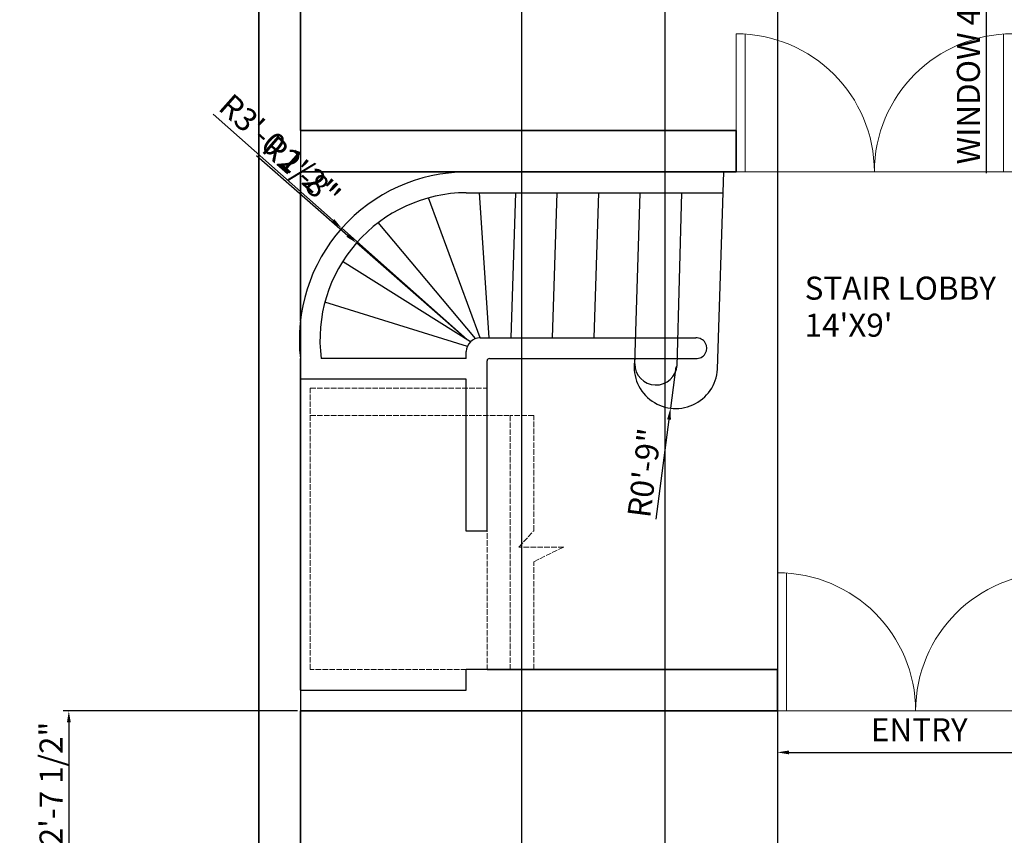
# Model space of a CAD drawing. Units: inches. Extents: x 1265 to 2734, y 1741 to 2595.
# Tile 2 of 10: x 2277 to 2490, y 1988 to 2165. Entities that reach past the tile are written whole.
import ezdxf

# ---------------------------------------------------------------- set-up
doc = ezdxf.new("R2010")
doc.units = ezdxf.units.IN
doc.header["$LTSCALE"] = 0.1
doc.linetypes.add('ACAD_ISO02W100', pattern=[15, 12, -3])
for name, color, linetype, lineweight in [('A-ANNO-DIMS', 2, 'Continuous', 18), ('A-ANNO-TEXT', 7, 'Continuous', 18), ('A-AREA-IDEN', 7, 'Continuous', 18), ('A-DOOR', 3, 'Continuous', 18), ('A-FLOR-STRS', 7, 'Continuous', 25), ('A-FLOR-STRS-HIDN', 8, 'ACAD_ISO02W100', 18), ('A-WALL', 7, 'Continuous', 35), ('C-PROP', 7, 'Continuous', 35), ('L-HRDS', 8, 'Continuous', 25)]:
    doc.layers.add(name, color=color, linetype=linetype, lineweight=lineweight)
doc.styles.get("Standard").update_dxf_attribs({"font": 'arial.ttf', "height": 5})
doc.dimstyles.new('ISO-25', dxfattribs={"dimtxt": 5, "dimasz": 2.5, "dimexe": 1.25, "dimexo": 0.625, "dimtad": 1, "dimlunit": 3, "dimtxsty": 'Standard', "dimcen": 2.5, "dimadec": 0, "dimazin": 0, "dimtfac": 1, "dimtmove": 0, "dimatfit": 3, "dimfxl": 1, "dimarcsym": 0})

# ---------------------------------------------------------------- blocks, each defined once
blk = doc.blocks.new('DOOR-PAIR-60IN')
for p, q in [((0, 30), (0, 0)), ((2, 29.93), (2, 0)), ((58, 29.93), (58, 0)), ((60, 30), (60, 0)), ((0, 0), (30, 0)), ((60, 0), (30, 0))]:
    blk.add_line(p, q)
for centre, start, end in [((0, 0), 0, 90), ((60, 0), 90, 180)]:
    blk.add_arc(centre, 30, start, end)
blk = doc.blocks.new('*D34')
at = {"layer": 'A-ANNO-DIMS', "color": 0, "lineweight": -2, "transparency": 16777216}
for p, q in [((2441.1, 2014.03), (2441.1, 2004.41)), ((2501.1, 2014.03), (2501.1, 2004.41)), ((2443.6, 2005.66), (2498.6, 2005.66)), ((2501.1, 2005.66), (2588.64, 2005.66))]:
    blk.add_line(p, q, dxfattribs=at)
at = {"layer": 'A-ANNO-DIMS', "color": 0, "lineweight": 100, "transparency": 16777216}
for points in [[(2443.6, 2006.07), (2443.6, 2005.24), (2441.1, 2005.66)], [(2498.6, 2006.07), (2498.6, 2005.24), (2501.1, 2005.66)]]:
    blk.add_solid(points, dxfattribs=at)
at = {"layer": 'Defpoints', "color": 0, "lineweight": 100, "transparency": 16777216}
for p in [(2441.1, 2014.66), (2501.1, 2014.66), (2501.1, 2005.66)]:
    blk.add_point(p, dxfattribs=at)
at = {"layer": 'A-ANNO-DIMS', "color": 0, "transparency": 16777216, "insert": (2546.12, 2008.87), "char_height": 5, "attachment_point": 5}
blk.add_mtext('DOUBLE DOOR 5\'-0" TYP.', dxfattribs=at)
blk = doc.blocks.new('*D36')
at = {"layer": 'A-ANNO-DIMS', "color": 0, "lineweight": -2, "transparency": 16777216}
for p, q in [((2492.98, 2246.41), (2485.15, 2246.41)), ((2486.4, 2243.91), (2486.4, 2200.91)), ((2492.98, 2198.41), (2485.15, 2198.41)), ((2486.4, 2198.41), (2486.4, 2131.39))]:
    blk.add_line(p, q, dxfattribs=at)
at = {"layer": 'A-ANNO-DIMS', "color": 0, "lineweight": 100, "transparency": 16777216}
for points in [[(2485.99, 2243.91), (2486.82, 2243.91), (2486.4, 2246.41)], [(2485.99, 2200.91), (2486.82, 2200.91), (2486.4, 2198.41)]]:
    blk.add_solid(points, dxfattribs=at)
at = {"layer": 'Defpoints', "color": 0, "lineweight": 100, "transparency": 16777216}
for p in [(2493.6, 2246.41), (2486.4, 2198.41), (2493.6, 2198.41)]:
    blk.add_point(p, dxfattribs=at)
at = {"layer": 'A-ANNO-DIMS', "color": 0, "transparency": 16777216, "insert": (2483.19, 2163.65), "char_height": 5, "attachment_point": 5, "rotation": 90}
blk.add_mtext('WINDOW 4\'-0" TYP.', dxfattribs=at)
blk = doc.blocks.new('*D41')
at = {"layer": 'A-ANNO-DIMS', "color": 0, "lineweight": -2, "transparency": 16777216}
for p, q in [((2336.98, 2014.66), (2286.1, 2014.66)), ((2287.35, 2012.16), (2287.35, 1985.66)), ((2504.98, 1983.16), (2286.1, 1983.16))]:
    blk.add_line(p, q, dxfattribs=at)
at = {"layer": 'A-ANNO-DIMS', "color": 0, "lineweight": 100, "transparency": 16777216}
for points in [[(2286.94, 2012.16), (2287.77, 2012.16), (2287.35, 2014.66)], [(2286.94, 1985.66), (2287.77, 1985.66), (2287.35, 1983.16)]]:
    blk.add_solid(points, dxfattribs=at)
at = {"layer": 'Defpoints', "color": 0, "lineweight": 100, "transparency": 16777216}
for p in [(2337.6, 2014.66), (2287.35, 1983.16), (2505.6, 1983.16)]:
    blk.add_point(p, dxfattribs=at)
at = {"layer": 'A-ANNO-DIMS', "color": 0, "transparency": 16777216, "insert": (2284.14, 1998.91), "char_height": 5, "attachment_point": 5, "rotation": 90}
blk.add_mtext('2\'-7 1/2"', dxfattribs=at)
blk = doc.blocks.new('*D42')
at = {"layer": 'A-ANNO-DIMS', "color": 0, "lineweight": -2, "transparency": 16777216}
for p, q in [((2328.6, 1822.68), (2328.6, 2585.16)), ((2331.1, 2583.91), (2518.82, 2583.91)), ((2521.32, 1822.68), (2521.32, 2585.16))]:
    blk.add_line(p, q, dxfattribs=at)
at = {"layer": 'A-ANNO-DIMS', "color": 0, "lineweight": 100, "transparency": 16777216}
for points in [[(2331.1, 2584.32), (2331.1, 2583.49), (2328.6, 2583.91)], [(2518.82, 2584.32), (2518.82, 2583.49), (2521.32, 2583.91)]]:
    blk.add_solid(points, dxfattribs=at)
at = {"layer": 'Defpoints', "color": 0, "lineweight": 100, "transparency": 16777216}
for p in [(2521.32, 2583.91), (2328.6, 1822.06), (2521.32, 1822.06)]:
    blk.add_point(p, dxfattribs=at)
at = {"layer": 'A-ANNO-DIMS', "color": 0, "transparency": 16777216, "insert": (2424.96, 2587.12), "char_height": 5, "attachment_point": 5}
blk.add_mtext('16\'-0 1/2"', dxfattribs=at)
blk = doc.blocks.new('*D43')
at = {"layer": 'A-ANNO-DIMS', "color": 0, "lineweight": -2, "transparency": 16777216}
for p, q in [((2337.6, 2308.03), (2337.6, 1744.16)), ((2441.1, 2308.03), (2441.1, 1744.16)), ((2340.1, 1745.41), (2438.6, 1745.41))]:
    blk.add_line(p, q, dxfattribs=at)
at = {"layer": 'A-ANNO-DIMS', "color": 0, "lineweight": 100, "transparency": 16777216}
for points in [[(2340.1, 1745.82), (2340.1, 1744.99), (2337.6, 1745.41)], [(2438.6, 1745.82), (2438.6, 1744.99), (2441.1, 1745.41)]]:
    blk.add_solid(points, dxfattribs=at)
at = {"layer": 'Defpoints', "color": 0, "lineweight": 100, "transparency": 16777216}
for p in [(2337.6, 2308.66), (2441.1, 2308.66), (2441.1, 1745.41)]:
    blk.add_point(p, dxfattribs=at)
at = {"layer": 'A-ANNO-DIMS', "color": 0, "transparency": 16777216, "insert": (2389.35, 1748.62), "char_height": 5, "attachment_point": 5}
blk.add_mtext('8\'-7 1/2"', dxfattribs=at)
blk = doc.blocks.new('*D45')
at = {"layer": 'A-ANNO-DIMS', "color": 0, "lineweight": -2, "transparency": 16777216}
for p, q in [((2385.6, 2477.53), (2385.6, 1744.16)), ((2416.67, 2477.91), (2416.67, 1744.16)), ((2388.1, 1745.41), (2414.17, 1745.41))]:
    blk.add_line(p, q, dxfattribs=at)
at = {"layer": 'A-ANNO-DIMS', "color": 0, "lineweight": 100, "transparency": 16777216}
for points in [[(2388.1, 1745.82), (2388.1, 1744.99), (2385.6, 1745.41)], [(2414.17, 1745.82), (2414.17, 1744.99), (2416.67, 1745.41)]]:
    blk.add_solid(points, dxfattribs=at)
at = {"layer": 'Defpoints', "color": 0, "lineweight": 100, "transparency": 16777216}
for p in [(2416.67, 2478.54), (2385.6, 2478.16), (2416.67, 1745.41)]:
    blk.add_point(p, dxfattribs=at)
at = {"layer": 'A-ANNO-DIMS', "color": 0, "transparency": 16777216, "insert": (2401.14, 1748.54), "char_height": 5, "attachment_point": 5}
blk.add_mtext('2\'-7"', dxfattribs=at)
blk = doc.blocks.new('*D48')
at = {"layer": 'A-ANNO-DIMS', "color": 0, "lineweight": -2, "transparency": 16777216}
for p, q in [((2337.6, 2014.03), (2337.6, 1744.16)), ((2441.1, 2014.03), (2441.1, 1744.16)), ((2340.1, 1745.41), (2438.6, 1745.41))]:
    blk.add_line(p, q, dxfattribs=at)
at = {"layer": 'A-ANNO-DIMS', "color": 0, "lineweight": 100, "transparency": 16777216}
for points in [[(2340.1, 1745.82), (2340.1, 1744.99), (2337.6, 1745.41)], [(2438.6, 1745.82), (2438.6, 1744.99), (2441.1, 1745.41)]]:
    blk.add_solid(points, dxfattribs=at)
at = {"layer": 'Defpoints', "color": 0, "lineweight": 100, "transparency": 16777216}
for p in [(2337.6, 2014.66), (2441.1, 2014.66), (2441.1, 1745.41)]:
    blk.add_point(p, dxfattribs=at)
at = {"layer": 'A-ANNO-DIMS', "color": 0, "transparency": 16777216, "insert": (2389.35, 1748.62), "char_height": 5, "attachment_point": 5}
blk.add_mtext('8\'-7 1/2"', dxfattribs=at)
blk = doc.blocks.new('*D50')
at = {"layer": 'A-ANNO-DIMS', "color": 0, "lineweight": -2, "transparency": 16777216}
for p, q in [((2318.67, 2144.24), (2344.7, 2121.1)), ((2373.77, 2095.26), (2346.56, 2119.44))]:
    blk.add_line(p, q, dxfattribs=at)
at = {"layer": 'A-ANNO-DIMS', "color": 0, "lineweight": 100, "transparency": 16777216}
blk.add_solid([(2344.97, 2121.41), (2344.42, 2120.79), (2346.56, 2119.44)], dxfattribs=at)
at = {"layer": 'Defpoints', "color": 0, "lineweight": 100, "transparency": 16777216}
for p in [(2346.56, 2119.44), (2373.77, 2095.26)]:
    blk.add_point(p, dxfattribs=at)
at = {"layer": 'A-ANNO-DIMS', "color": 0, "transparency": 16777216, "insert": (2332.38, 2136.35), "char_height": 5, "attachment_point": 5, "rotation": 318.3664}
blk.add_mtext('R3\'-0 1/2"', dxfattribs=at)
blk = doc.blocks.new('*D51')
at = {"layer": 'A-ANNO-DIMS', "color": 0, "lineweight": -2, "transparency": 16777216}
for p, q in [((2328.05, 2135.23), (2347.87, 2117.9)), ((2373.79, 2095.22), (2349.75, 2116.25))]:
    blk.add_line(p, q, dxfattribs=at)
at = {"layer": 'A-ANNO-DIMS', "color": 0, "lineweight": 100, "transparency": 16777216}
blk.add_solid([(2348.14, 2118.21), (2347.59, 2117.58), (2349.75, 2116.25)], dxfattribs=at)
at = {"layer": 'Defpoints', "color": 0, "lineweight": 100, "transparency": 16777216}
for p in [(2349.75, 2116.25), (2373.79, 2095.22)]:
    blk.add_point(p, dxfattribs=at)
at = {"layer": 'A-ANNO-DIMS', "color": 0, "transparency": 16777216, "insert": (2337.42, 2131.26), "char_height": 5, "attachment_point": 5, "rotation": 318.8141}
blk.add_mtext('R2\'-8"', dxfattribs=at)
blk = doc.blocks.new('*D52')
at = {"layer": 'A-ANNO-DIMS', "color": 0, "lineweight": -2, "transparency": 16777216}
for p, q in [((2419.06, 2089.38), (2417.9, 2080.39)), ((2414.8, 2056.26), (2417.59, 2077.91))]:
    blk.add_line(p, q, dxfattribs=at)
at = {"layer": 'A-ANNO-DIMS', "color": 0, "lineweight": 100, "transparency": 16777216}
blk.add_solid([(2417.17, 2077.96), (2418, 2077.86), (2417.9, 2080.39)], dxfattribs=at)
at = {"layer": 'Defpoints', "color": 0, "lineweight": 100, "transparency": 16777216}
for p in [(2419.06, 2089.38), (2417.9, 2080.39)]:
    blk.add_point(p, dxfattribs=at)
at = {"layer": 'A-ANNO-DIMS', "color": 0, "transparency": 16777216, "insert": (2412.88, 2066.25), "char_height": 5, "attachment_point": 5, "rotation": 82.6604}
blk.add_mtext('R0\'-9"', dxfattribs=at)

msp = doc.modelspace()

# ---------------------------------------------------------------- linework, layer by layer
at = {"layer": 'A-FLOR-STRS'}
for p, q in [((2337.602, 2099.365), (2337.602, 2131.657)), ((2428.111, 2088.847), (2429.486, 2131.657)), ((2376.602, 2095.657), (2365.364, 2126.027)), ((2373.602, 2127.157), (2429.342, 2127.157)), ((2378.534, 2095.657), (2376.437, 2127.157)), ((2383.306, 2095.657), (2384.318, 2127.157)), ((2392.311, 2095.657), (2393.323, 2127.157)), ((2401.315, 2095.657), (2402.328, 2127.157)), ((2410.139, 2090.017), (2411.332, 2127.157)), ((2419.325, 2089.47), (2420.337, 2127.157)), ((2375.601, 2095.485), (2354.489, 2120.67)), ((2374.481, 2094.778), (2346.744, 2112.217)), ((2373.824, 2093.788), (2342.917, 2103.426)), ((2376.602, 2095.657), (2423.408, 2095.657)), ((2373.602, 2091.157), (2373.602, 2092.657)), ((2337.602, 2019.157), (2337.602, 2091.157)), ((2373.602, 2091.157), (2342.102, 2091.157)), ((2378.102, 2053.657), (2378.102, 2090.657)), ((2378.602, 2091.157), (2423.661, 2091.157)), ((2373.602, 2086.657), (2337.602, 2086.657)), ((2373.602, 2053.657), (2373.602, 2086.657)), ((2378.102, 2053.657), (2373.602, 2053.657)), ((2373.602, 2019.157), (2373.602, 2023.657)), ((2378.102, 2023.657), (2373.602, 2023.657)), ((2337.602, 2019.157), (2373.602, 2019.157))]:
    msp.add_line(p, q, dxfattribs=at)
for centre, radius, start, end in [((2373.766, 2095.261), 36.396, 90.25802, 186.4749), ((2373.785, 2095.216), 31.942, 90.32776, 187.30039), ((2376.602, 2092.657), 3, 90, 180), ((2423.534, 2093.407), 2.254, 266.77563, 93.22437), ((2378.602, 2090.657), 0.5, 90, 180), ((2419.063, 2089.379), 9.063, 168.68911, 356.6316), ((2414.739, 2090.017), 4.6, 180, 356.92292)]:
    msp.add_arc(centre, radius, start, end, dxfattribs=at)
at = {"layer": 'A-FLOR-STRS-HIDN'}
for p, q in [((2339.725, 2084.719), (2378.102, 2084.719)), ((2339.725, 2023.657), (2339.725, 2084.719)), ((2378.102, 2084.719), (2378.102, 2023.657)), ((2339.725, 2078.788), (2383.147, 2078.788)), ((2383.147, 2078.788), (2383.147, 2023.657)), ((2388.226, 2078.788), (2383.147, 2078.788)), ((2388.226, 2053.768), (2388.226, 2078.788)), ((2385.029, 2050.244), (2388.226, 2053.768)), ((2394.73, 2050.244), (2385.029, 2050.244)), ((2388.226, 2047.049), (2394.73, 2050.244)), ((2388.226, 2023.657), (2388.226, 2047.049)), ((2378.102, 2023.657), (2339.725, 2023.657)), ((2383.147, 2023.657), (2378.102, 2023.657)), ((2383.147, 2023.657), (2388.226, 2023.657))]:
    msp.add_line(p, q, dxfattribs=at)
at = {"layer": 'A-WALL'}
for p, q in [((2337.602, 2140.657), (2337.602, 2308.657)), ((2337.602, 2140.657), (2432.143, 2140.657)), ((2432.143, 2140.657), (2432.143, 2131.657)), ((2337.602, 2131.657), (2432.143, 2131.657)), ((2378.102, 2023.657), (2441.102, 2023.657)), ((2441.102, 2023.657), (2441.102, 2014.657)), ((2337.602, 2014.657), (2441.102, 2014.657))]:
    msp.add_line(p, q, dxfattribs=at)
at = {"layer": 'C-PROP'}
msp.add_line((2328.602, 1786.657), (2328.602, 2542.657), dxfattribs=at)
at = {"layer": 'L-HRDS'}
msp.add_line((2337.602, 1822.059), (2337.602, 2014.657), dxfattribs=at)

# ---------------------------------------------------------------- block references
at = {"layer": 'A-DOOR'}
for p in [(2432.143, 2131.657), (2441.103, 2014.657)]:
    msp.add_blockref('DOOR-PAIR-60IN', p, dxfattribs=at)

# ---------------------------------------------------------------- texts
at = {"layer": 'A-ANNO-TEXT'}
msp.add_text('ENTRY', height=5, dxfattribs=at).set_placement((2461.412, 2008.066))
at = {"layer": 'A-AREA-IDEN'}
for s, p in [('STAIR LOBBY', (2447.028, 2103.939)), ("14'X9'", (2447.028, 2095.906))]:
    msp.add_text(s, height=5, dxfattribs=at).set_placement(p)

# ---------------------------------------------------------------- dimensions: what is measured, and where the dimension line sits
at = {"layer": 'A-ANNO-DIMS'}
for base, p1, p2, picture, middle in [((2521.319, 2583.907), (2328.602, 1822.059), (2521.319, 1822.059), '*D42', (2424.961, 2587.117)), ((2416.673, 1745.407), (2385.602, 2478.157), (2416.673, 2478.538), '*D45', (2401.138, 1748.542)), ((2441.102, 1745.407), (2337.602, 2308.657), (2441.102, 2308.657), '*D43', (2389.352, 1748.617)), ((2441.102, 1745.407), (2337.602, 2014.657), (2441.102, 2014.657), '*D48', (2389.352, 1748.617))]:
    dim = msp.add_linear_dim(base=base, p1=p1, p2=p2, dimstyle='ISO-25', override={"dimdec": 1, "dimlfac": 1, "dimrnd": 0, "dimzin": 1, "dimdsep": 46, "dimlunit": 4, "dimfrac": 2}, dxfattribs=at)
    dim.commit()
    dim.dimension.update_dxf_attribs({"geometry": picture, "text_midpoint": middle})
dim = msp.add_linear_dim(base=(2486.402, 2198.407), p1=(2493.602, 2246.407), p2=(2493.602, 2198.407), angle=270, text='WINDOW <> TYP.', dimstyle='ISO-25', override={"dimdec": 1, "dimlfac": 1, "dimrnd": 0, "dimzin": 1, "dimdsep": 46, "dimlunit": 4, "dimfrac": 2}, dxfattribs=at)
dim.commit()
dim.dimension.update_dxf_attribs({"geometry": '*D36', "text_midpoint": (2483.19, 2163.646)})
for center, mpoint, picture, middle in [((2373.766, 2095.261), (2346.564, 2119.441), '*D50', (2330.242, 2133.949)), ((2373.785, 2095.216), (2349.747, 2116.249), '*D51', (2335.324, 2128.87))]:
    dim = msp.add_radius_dim(center=center, mpoint=mpoint, dimstyle='ISO-25', override={"dimdec": 1, "dimlfac": 1, "dimrnd": 0, "dimzin": 1, "dimdsep": 46, "dimlunit": 4, "dimfrac": 2}, dxfattribs=at)
    dim.commit()
    dim.dimension.update_dxf_attribs({"geometry": picture, "text_midpoint": middle, "dimtype": 164})
dim = msp.add_radius_dim(center=(2419.063, 2089.379), mpoint=(2417.905, 2080.39), dimstyle='ISO-25', override={"dimdec": 1, "dimlfac": 1, "dimrnd": 0, "dimzin": 1, "dimdsep": 46, "dimlunit": 4, "dimfrac": 2}, dxfattribs=at)
dim.commit()
dim.dimension.update_dxf_attribs({"geometry": '*D52', "text_midpoint": (2412.88, 2066.253)})
dim = msp.add_linear_dim(base=(2501.102, 2005.657), p1=(2441.102, 2014.657), p2=(2501.102, 2014.657), text='DOUBLE DOOR <> TYP.', dimstyle='ISO-25', override={"dimdec": 1, "dimlfac": 1, "dimrnd": 0, "dimzin": 1, "dimdsep": 46, "dimlunit": 4, "dimfrac": 2}, dxfattribs=at)
dim.commit()
dim.dimension.update_dxf_attribs({"geometry": '*D34', "text_midpoint": (2546.122, 2008.869)})
dim = msp.add_linear_dim(base=(2287.352, 1983.157), p1=(2337.602, 2014.657), p2=(2505.602, 1983.157), angle=90, dimstyle='ISO-25', override={"dimdec": 1, "dimlfac": 1, "dimrnd": 0, "dimzin": 1, "dimdsep": 46, "dimlunit": 4, "dimfrac": 2}, dxfattribs=at)
dim.commit()
dim.dimension.update_dxf_attribs({"geometry": '*D41', "text_midpoint": (2284.142, 1998.907)})

doc.saveas('drawing.dxf')
